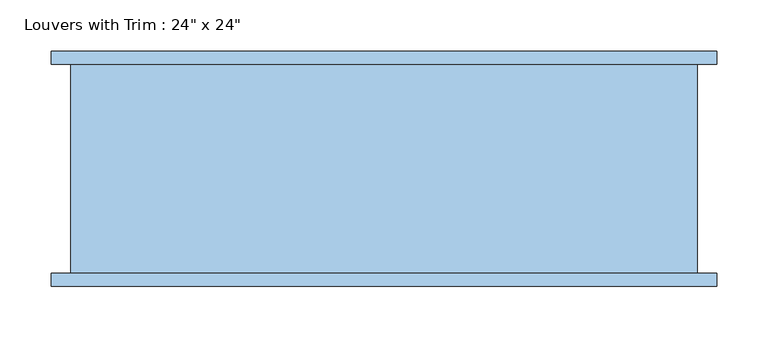
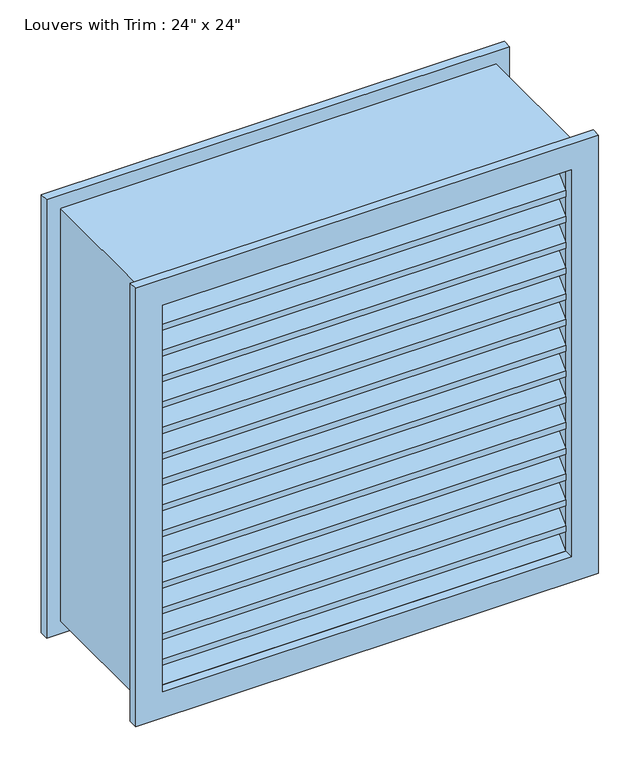
"""IFC4 building model written with IfcOpenShell, lengths in millimetres: window geometry."""

from ifc_helpers import new_model, si_unit, frame, origin, place, context, project, spatial, polyline, outline, extrude, source, transform, mapped, element, save


def window_75debfae(model_context):
    return source(origin(), model_context, "Body", "SweptSolid", [
        extrude(outline(polyline([(1543.05, -323.85), (895.35, -323.85), (895.35, 323.85), (1543.05, 323.85), (1543.05, -323.85)]), holes=[polyline([(1504.95, -285.75), (1504.95, 285.75), (933.45, 285.75), (933.45, -285.75), (1504.95, -285.75)])]), frame((0.0, -107.95, 0.0), z_axis=(0.0, 1.0, 0.0), x_axis=(0.0, 0.0, 1.0)), (0.0, 0.0, 1.0), 12.7),
        extrude(outline(polyline([(1543.05, 323.85), (1543.05, -323.85), (895.35, -323.85), (895.35, 323.85), (1543.05, 323.85)]), holes=[polyline([(1504.95, 285.75), (933.45, 285.75), (933.45, -285.75), (1504.95, -285.75), (1504.95, 285.75)])]), frame((0.0, 107.95, 0.0), z_axis=(0.0, 1.0, 0.0), x_axis=(0.0, 0.0, 1.0)), (0.0, 0.0, 1.0), 12.7),
        extrude(outline(polyline([(1524.0, 304.8), (1524.0, -304.8), (914.4, -304.8), (914.4, 304.8), (1524.0, 304.8)]), holes=[polyline([(1504.95, 285.75), (933.45, 285.75), (933.45, -285.75), (1504.95, -285.75), (1504.95, 285.75)])]), frame((0.0, -95.25, 0.0), z_axis=(0.0, 1.0, 0.0), x_axis=(0.0, 0.0, 1.0)), (0.0, 0.0, 1.0), 203.2),
        extrude(outline(polyline([(-59.3289755, 969.3710245), (-23.407951, 933.45), (-32.3882072, 933.45), (-59.3289755, 960.3907684), (-86.2697439, 933.45), (-95.25, 933.45), (-59.3289755, 969.3710245)])), frame((-285.75, 0.0, 0.0), z_axis=(1.0, 0.0, 0.0), x_axis=(0.0, 1.0, 0.0)), (0.0, 0.0, 1.0), 571.5),
        extrude(outline(polyline([(-59.3289755, 1007.4710245), (-23.407951, 971.55), (-23.407951, 962.5697439), (-59.3289755, 998.4907684), (-95.25, 962.5697439), (-95.25, 971.55), (-59.3289755, 1007.4710245)])), frame((-285.75, 0.0, 0.0), z_axis=(1.0, 0.0, 0.0), x_axis=(0.0, 1.0, 0.0)), (0.0, 0.0, 1.0), 571.5),
        extrude(outline(polyline([(-59.3289755, 1045.5710245), (-23.407951, 1009.65), (-23.407951, 1000.6697439), (-59.3289755, 1036.5907684), (-95.25, 1000.6697439), (-95.25, 1009.65), (-59.3289755, 1045.5710245)])), frame((-285.75, 0.0, 0.0), z_axis=(1.0, 0.0, 0.0), x_axis=(0.0, 1.0, 0.0)), (0.0, 0.0, 1.0), 571.5),
        extrude(outline(polyline([(-59.3289755, 1083.6710245), (-23.407951, 1047.75), (-23.407951, 1038.7697439), (-59.3289755, 1074.6907684), (-95.25, 1038.7697439), (-95.25, 1047.75), (-59.3289755, 1083.6710245)])), frame((-285.75, 0.0, 0.0), z_axis=(1.0, 0.0, 0.0), x_axis=(0.0, 1.0, 0.0)), (0.0, 0.0, 1.0), 571.5),
        extrude(outline(polyline([(-59.3289755, 1121.7710245), (-23.407951, 1085.85), (-23.407951, 1076.8697439), (-59.3289755, 1112.7907684), (-95.25, 1076.8697439), (-95.25, 1085.85), (-59.3289755, 1121.7710245)])), frame((-285.75, 0.0, 0.0), z_axis=(1.0, 0.0, 0.0), x_axis=(0.0, 1.0, 0.0)), (0.0, 0.0, 1.0), 571.5),
        extrude(outline(polyline([(-59.3289755, 1159.8710245), (-23.407951, 1123.95), (-23.407951, 1114.9697439), (-59.3289755, 1150.8907684), (-95.25, 1114.9697439), (-95.25, 1123.95), (-59.3289755, 1159.8710245)])), frame((-285.75, 0.0, 0.0), z_axis=(1.0, 0.0, 0.0), x_axis=(0.0, 1.0, 0.0)), (0.0, 0.0, 1.0), 571.5),
        extrude(outline(polyline([(-59.3289755, 1197.9710245), (-23.407951, 1162.05), (-23.407951, 1153.0697439), (-59.3289755, 1188.9907684), (-95.25, 1153.0697439), (-95.25, 1162.05), (-59.3289755, 1197.9710245)])), frame((-285.75, 0.0, 0.0), z_axis=(1.0, 0.0, 0.0), x_axis=(0.0, 1.0, 0.0)), (0.0, 0.0, 1.0), 571.5),
        extrude(outline(polyline([(-59.3289755, 1236.0710245), (-23.407951, 1200.15), (-23.407951, 1191.1697439), (-59.3289755, 1227.0907684), (-95.25, 1191.1697439), (-95.25, 1200.15), (-59.3289755, 1236.0710245)])), frame((-285.75, 0.0, 0.0), z_axis=(1.0, 0.0, 0.0), x_axis=(0.0, 1.0, 0.0)), (0.0, 0.0, 1.0), 571.5),
        extrude(outline(polyline([(-59.3289755, 1274.1710245), (-23.407951, 1238.25), (-23.407951, 1229.2697439), (-59.3289755, 1265.1907684), (-95.25, 1229.2697439), (-95.25, 1238.25), (-59.3289755, 1274.1710245)])), frame((-285.75, 0.0, 0.0), z_axis=(1.0, 0.0, 0.0), x_axis=(0.0, 1.0, 0.0)), (0.0, 0.0, 1.0), 571.5),
        extrude(outline(polyline([(-59.3289755, 1312.2710245), (-23.407951, 1276.35), (-23.407951, 1267.3697439), (-59.3289755, 1303.2907684), (-95.25, 1267.3697439), (-95.25, 1276.35), (-59.3289755, 1312.2710245)])), frame((-285.75, 0.0, 0.0), z_axis=(1.0, 0.0, 0.0), x_axis=(0.0, 1.0, 0.0)), (0.0, 0.0, 1.0), 571.5),
        extrude(outline(polyline([(-59.3289755, 1350.3710245), (-23.407951, 1314.45), (-23.407951, 1305.4697439), (-59.3289755, 1341.3907684), (-95.25, 1305.4697439), (-95.25, 1314.45), (-59.3289755, 1350.3710245)])), frame((-285.75, 0.0, 0.0), z_axis=(1.0, 0.0, 0.0), x_axis=(0.0, 1.0, 0.0)), (0.0, 0.0, 1.0), 571.5),
        extrude(outline(polyline([(-59.3289755, 1388.4710245), (-23.407951, 1352.55), (-23.407951, 1343.5697439), (-59.3289755, 1379.4907684), (-95.25, 1343.5697439), (-95.25, 1352.55), (-59.3289755, 1388.4710245)])), frame((-285.75, 0.0, 0.0), z_axis=(1.0, 0.0, 0.0), x_axis=(0.0, 1.0, 0.0)), (0.0, 0.0, 1.0), 571.5),
        extrude(outline(polyline([(-59.3289755, 1426.5710245), (-23.407951, 1390.65), (-23.407951, 1381.6697439), (-59.3289755, 1417.5907684), (-95.25, 1381.6697439), (-95.25, 1390.65), (-59.3289755, 1426.5710245)])), frame((-285.75, 0.0, 0.0), z_axis=(1.0, 0.0, 0.0), x_axis=(0.0, 1.0, 0.0)), (0.0, 0.0, 1.0), 571.5),
        extrude(outline(polyline([(-59.3289755, 1464.6710245), (-23.407951, 1428.75), (-23.407951, 1419.7697439), (-59.3289755, 1455.6907684), (-95.25, 1419.7697439), (-95.25, 1428.75), (-59.3289755, 1464.6710245)])), frame((-285.75, 0.0, 0.0), z_axis=(1.0, 0.0, 0.0), x_axis=(0.0, 1.0, 0.0)), (0.0, 0.0, 1.0), 571.5),
        extrude(outline(polyline([(-59.3289755, 1502.7710245), (-23.407951, 1466.85), (-23.407951, 1457.8697439), (-59.3289755, 1493.7907684), (-95.25, 1457.8697439), (-95.25, 1466.85), (-59.3289755, 1502.7710245)])), frame((-285.75, 0.0, 0.0), z_axis=(1.0, 0.0, 0.0), x_axis=(0.0, 1.0, 0.0)), (0.0, 0.0, 1.0), 571.5),
    ])


if __name__ == "__main__":
    model = new_model("IFC4")
    model_context = context("Model", 3, world=origin())
    ifc_project = project(units=[si_unit("LENGTHUNIT", "METRE", prefix="MILLI")], contexts=[model_context])
    site = spatial("IfcSite", under=ifc_project)
    building = spatial("IfcBuilding", under=site)
    placement = place(None, origin())
    window_shape = window_75debfae(model_context)
    element("IfcWindow", 1, ObjectType="Louvers with Trim : 24\" x 24\"", at=placement, inside=building, context=model_context, shape_type="MappedRepresentation", body=[
        mapped(window_shape, transform((0.0, 0.0, 0.0), x_axis=(1.0, 0.0, 0.0), y_axis=(0.0, 1.0, 0.0), z_axis=(0.0, 0.0, 1.0))),
    ])
    save(model, "model.ifc")

# Revit data of these elements
# Type "Louvers with Trim : 24\" x 24\""
#   Type Mark = "10"
#   Construction Type Id = "GSP4R"
#   Assembly Code = "B20"
#   Analytic Construction = "1/8 in Pilkington single glazing"
#   Visual Light Transmittance = 0.9
#   Solar Heat Gain Coefficient = 0.78
#   Heat Transfer Coefficient (U) = 0.6496 BTU/(h·ft²·°F)
#   Default Sill Height = 3' - 0"
#   Trim Projection - Ext. = 0' - 0 1/2"
#   Trim Projection - Int. = 0' - 0 1/2"
#   Trim Width - Exterior = 0' - 1 1/2"
#   Trim Width - Interior = 0' - 1 1/2"
#   Width = 2' - 0"
#   Define Thermal Properties by = 1
#   Frame Material = Birch
#   Louver Material = Birch
#   Trim Exterior Material = Birch
#   Trim Interior Material = Birch
#   Wall Closure = (empty or 0)
# Element 1 (IfcWindow, "Louvers with Trim : 24\" x 24\"")
#   Materials on its faces: "Birch"
# Materials
#   "Birch": class "Wood", colour RGB 224 178 126, transparency 0, Description = "Betula Alleghaniensis", Cost = 0
